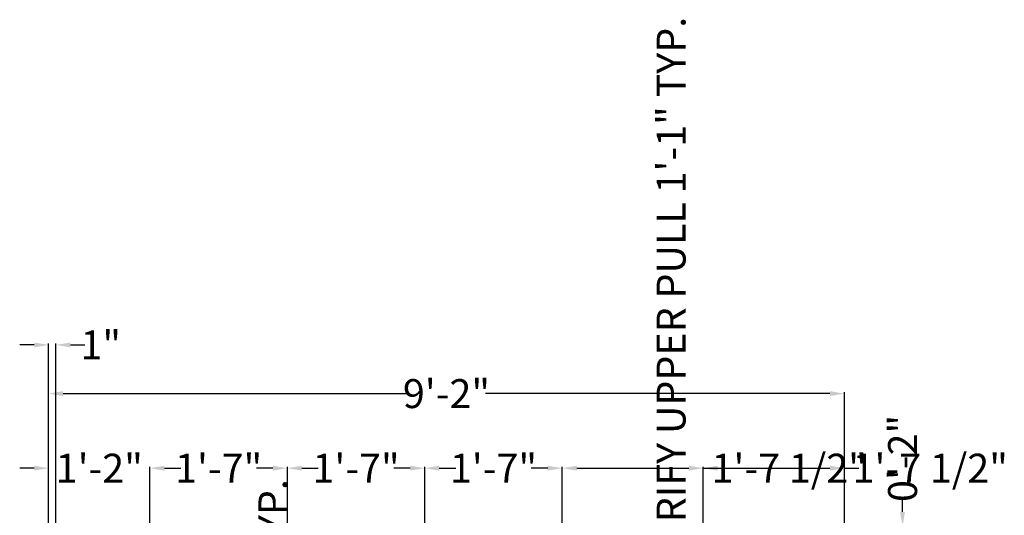
# Model space of a CAD drawing. Units: inches. Extents: x 13 to 156, y 156 to 357.
# Tile 3 of 3: x 20 to 156, y 289 to 357. Entities that reach past the tile are written whole.
import ezdxf

# ---------------------------------------------------------------- set-up
doc = ezdxf.new("R2010")
doc.units = ezdxf.units.IN
doc.header["$MEASUREMENT"] = 0
doc.layers.add('A-ANNO-DIMS', color=2, linetype='Continuous', lineweight=18)
doc.styles.get("Standard").update_dxf_attribs({"font": 'arial.ttf'})
doc.dimstyles.get("Standard").update_dxf_attribs({"dimtxt": 4, "dimasz": 2, "dimexe": 0.18, "dimexo": 0.0625, "dimgap": 0.09, "dimtad": 0, "dimdec": 0, "dimzin": 0, "dimdsep": 46, "dimlunit": 4, "dimtxsty": 'Standard', "dimcen": 0.09, "dimadec": 0, "dimazin": 0, "dimtfac": 1, "dimtdec": 0, "dimtofl": 0, "dimtmove": 0, "dimatfit": 3, "dimfxl": 1, "dimtolj": 1, "dimtzin": 0, "dimarcsym": 0})

# ---------------------------------------------------------------- blocks, each defined once
blk = doc.blocks.new('*D1')
at = {"layer": 'A-ANNO-DIMS', "color": 0, "lineweight": -2, "transparency": 16777216}
for p, q in [((23.63, 285.13), (23.63, 305.65)), ((25.63, 305.47), (73.22, 305.47)), ((131.63, 305.47), (84.03, 305.47)), ((133.63, 285.13), (133.63, 305.65))]:
    blk.add_line(p, q, dxfattribs=at)
at = {"layer": 'A-ANNO-DIMS', "color": 0, "transparency": 16777216}
for points in [[(25.63, 305.81), (25.63, 305.14), (23.63, 305.47)], [(131.63, 305.81), (131.63, 305.14), (133.63, 305.47)]]:
    blk.add_solid(points, dxfattribs=at)
at = {"layer": 'Defpoints', "color": 0, "transparency": 16777216}
for p in [(133.63, 305.47), (23.63, 285.07), (133.63, 285.07)]:
    blk.add_point(p, dxfattribs=at)
at = {"layer": 'A-ANNO-DIMS', "color": 0, "transparency": 16777216, "insert": (78.63, 305.47), "char_height": 4, "attachment_point": 5}
blk.add_mtext('\\A1;9\'-2"', dxfattribs=at)
blk = doc.blocks.new('*D2')
at = {"layer": 'A-ANNO-DIMS', "color": 0, "lineweight": -2, "transparency": 16777216}
for p, q in [((21.63, 312.2), (19.63, 312.2)), ((23.63, 285.13), (23.63, 312.38)), ((24.63, 285.13), (24.63, 312.38)), ((26.63, 312.2), (28.63, 312.2))]:
    blk.add_line(p, q, dxfattribs=at)
at = {"layer": 'A-ANNO-DIMS', "color": 0, "transparency": 16777216}
for points in [[(21.63, 312.54), (21.63, 311.87), (23.63, 312.2)], [(26.63, 312.54), (26.63, 311.87), (24.63, 312.2)]]:
    blk.add_solid(points, dxfattribs=at)
at = {"layer": 'Defpoints', "color": 0, "transparency": 16777216}
for p in [(24.63, 312.2), (23.63, 285.07), (24.63, 285.07)]:
    blk.add_point(p, dxfattribs=at)
at = {"layer": 'A-ANNO-DIMS', "color": 0, "transparency": 16777216, "insert": (30.83, 312.2), "char_height": 4, "attachment_point": 5}
blk.add_mtext('\\A1;1"', dxfattribs=at)
blk = doc.blocks.new('*D19')
at = {"layer": 'A-ANNO-DIMS', "color": 0, "lineweight": -2, "transparency": 16777216}
for p, q in [((109.68, 276.03), (109.68, 278.03)), ((111.56, 276.03), (109.5, 276.03)), ((109.68, 265.07), (109.68, 274.03)), ((111.56, 263.07), (109.5, 263.07))]:
    blk.add_line(p, q, dxfattribs=at)
at = {"layer": 'A-ANNO-DIMS', "color": 0, "transparency": 16777216}
for points in [[(109.35, 274.03), (110.01, 274.03), (109.68, 276.03)], [(109.35, 265.07), (110.01, 265.07), (109.68, 263.07)]]:
    blk.add_solid(points, dxfattribs=at)
at = {"layer": 'Defpoints', "color": 0, "transparency": 16777216}
for p in [(109.68, 276.03), (111.62, 276.03), (111.62, 263.07)]:
    blk.add_point(p, dxfattribs=at)
at = {"layer": 'A-ANNO-DIMS', "color": 0, "transparency": 16777216, "insert": (109.68, 319.45), "char_height": 4, "attachment_point": 5, "rotation": 90}
blk.add_mtext('\\A1;VERIFY UPPER PULL 1\'-1" TYP.', dxfattribs=at)
blk = doc.blocks.new('*D21')
at = {"layer": 'A-ANNO-DIMS', "color": 0, "lineweight": -2, "transparency": 16777216}
for p, q in [((54.63, 231.33), (54.63, 233.33)), ((58.13, 231.33), (54.45, 231.33)), ((54.63, 209.57), (54.63, 229.33)), ((58.13, 207.57), (54.45, 207.57))]:
    blk.add_line(p, q, dxfattribs=at)
at = {"layer": 'A-ANNO-DIMS', "color": 0, "transparency": 16777216}
for points in [[(54.29, 229.33), (54.96, 229.33), (54.63, 231.33)], [(54.29, 209.57), (54.96, 209.57), (54.63, 207.57)]]:
    blk.add_solid(points, dxfattribs=at)
at = {"layer": 'Defpoints', "color": 0, "transparency": 16777216}
for p in [(54.63, 231.33), (58.19, 231.33), (58.19, 207.57)]:
    blk.add_point(p, dxfattribs=at)
at = {"layer": 'A-ANNO-DIMS', "color": 0, "transparency": 16777216, "insert": (54.63, 264.31), "char_height": 4, "attachment_point": 5, "rotation": 90}
blk.add_mtext('\\A1;LOWER PULL 2\'-0" TYP.', dxfattribs=at)
blk = doc.blocks.new('*D31')
at = {"layer": 'A-ANNO-DIMS', "color": 0, "lineweight": -2, "transparency": 16777216}
for p, q in [((21.63, 295.16), (19.63, 295.16)), ((23.63, 285.13), (23.63, 295.34)), ((37.63, 285.13), (37.63, 295.34)), ((39.63, 295.16), (41.63, 295.16))]:
    blk.add_line(p, q, dxfattribs=at)
at = {"layer": 'A-ANNO-DIMS', "color": 0, "transparency": 16777216}
for points in [[(21.63, 295.49), (21.63, 294.82), (23.63, 295.16)], [(39.63, 295.49), (39.63, 294.82), (37.63, 295.16)]]:
    blk.add_solid(points, dxfattribs=at)
at = {"layer": 'Defpoints', "color": 0, "transparency": 16777216}
for p in [(37.63, 295.16), (23.63, 285.07), (37.63, 285.07)]:
    blk.add_point(p, dxfattribs=at)
at = {"layer": 'A-ANNO-DIMS', "color": 0, "transparency": 16777216, "insert": (30.63, 295.16), "char_height": 4, "attachment_point": 5}
blk.add_mtext('\\A1;1\'-2"', dxfattribs=at)
blk = doc.blocks.new('*D32')
at = {"layer": 'A-ANNO-DIMS', "color": 0, "lineweight": -2, "transparency": 16777216}
for p, q in [((37.63, 285.13), (37.63, 295.34)), ((39.63, 295.16), (41.91, 295.16)), ((54.63, 295.16), (52.35, 295.16)), ((56.63, 285.13), (56.63, 295.34))]:
    blk.add_line(p, q, dxfattribs=at)
at = {"layer": 'A-ANNO-DIMS', "color": 0, "transparency": 16777216}
for points in [[(39.63, 295.49), (39.63, 294.82), (37.63, 295.16)], [(54.63, 295.49), (54.63, 294.82), (56.63, 295.16)]]:
    blk.add_solid(points, dxfattribs=at)
at = {"layer": 'Defpoints', "color": 0, "transparency": 16777216}
for p in [(56.63, 295.16), (37.63, 285.07), (56.63, 285.07)]:
    blk.add_point(p, dxfattribs=at)
at = {"layer": 'A-ANNO-DIMS', "color": 0, "transparency": 16777216, "insert": (47.13, 295.16), "char_height": 4, "attachment_point": 5}
blk.add_mtext('\\A1;1\'-7"', dxfattribs=at)
blk = doc.blocks.new('*D33')
at = {"layer": 'A-ANNO-DIMS', "color": 0, "lineweight": -2, "transparency": 16777216}
for p, q in [((56.63, 285.13), (56.63, 295.34)), ((58.63, 295.16), (60.91, 295.16)), ((73.63, 295.16), (71.35, 295.16)), ((75.63, 285.13), (75.63, 295.34))]:
    blk.add_line(p, q, dxfattribs=at)
at = {"layer": 'A-ANNO-DIMS', "color": 0, "transparency": 16777216}
for points in [[(58.63, 295.49), (58.63, 294.82), (56.63, 295.16)], [(73.63, 295.49), (73.63, 294.82), (75.63, 295.16)]]:
    blk.add_solid(points, dxfattribs=at)
at = {"layer": 'Defpoints', "color": 0, "transparency": 16777216}
for p in [(75.63, 295.16), (56.63, 285.07), (75.63, 285.07)]:
    blk.add_point(p, dxfattribs=at)
at = {"layer": 'A-ANNO-DIMS', "color": 0, "transparency": 16777216, "insert": (66.13, 295.16), "char_height": 4, "attachment_point": 5}
blk.add_mtext('\\A1;1\'-7"', dxfattribs=at)
blk = doc.blocks.new('*D34')
at = {"layer": 'A-ANNO-DIMS', "color": 0, "lineweight": -2, "transparency": 16777216}
for p, q in [((75.63, 285.13), (75.63, 295.34)), ((77.63, 295.16), (79.91, 295.16)), ((92.63, 295.16), (90.35, 295.16)), ((94.63, 285.13), (94.63, 295.34))]:
    blk.add_line(p, q, dxfattribs=at)
at = {"layer": 'A-ANNO-DIMS', "color": 0, "transparency": 16777216}
for points in [[(77.63, 295.49), (77.63, 294.82), (75.63, 295.16)], [(92.63, 295.49), (92.63, 294.82), (94.63, 295.16)]]:
    blk.add_solid(points, dxfattribs=at)
at = {"layer": 'Defpoints', "color": 0, "transparency": 16777216}
for p in [(94.63, 295.16), (75.63, 285.07), (94.63, 285.07)]:
    blk.add_point(p, dxfattribs=at)
at = {"layer": 'A-ANNO-DIMS', "color": 0, "transparency": 16777216, "insert": (85.13, 295.16), "char_height": 4, "attachment_point": 5}
blk.add_mtext('\\A1;1\'-7"', dxfattribs=at)
blk = doc.blocks.new('*D35')
at = {"layer": 'A-ANNO-DIMS', "color": 0, "lineweight": -2, "transparency": 16777216}
for p, q in [((94.63, 285.13), (94.63, 295.34)), ((96.63, 295.16), (112.13, 295.16)), ((114.13, 285.13), (114.13, 295.34)), ((114.13, 295.16), (116.13, 295.16))]:
    blk.add_line(p, q, dxfattribs=at)
at = {"layer": 'A-ANNO-DIMS', "color": 0, "transparency": 16777216}
for points in [[(96.63, 295.49), (96.63, 294.82), (94.63, 295.16)], [(112.13, 295.49), (112.13, 294.82), (114.13, 295.16)]]:
    blk.add_solid(points, dxfattribs=at)
at = {"layer": 'Defpoints', "color": 0, "transparency": 16777216}
for p in [(114.13, 295.16), (94.63, 285.07), (114.13, 285.07)]:
    blk.add_point(p, dxfattribs=at)
at = {"layer": 'A-ANNO-DIMS', "color": 0, "transparency": 16777216, "insert": (126.01, 295.16), "char_height": 4, "attachment_point": 5}
blk.add_mtext('\\A1;1\'-7 1/2"', dxfattribs=at)
blk = doc.blocks.new('*D36')
at = {"layer": 'A-ANNO-DIMS', "color": 0, "lineweight": -2, "transparency": 16777216}
for p, q in [((114.13, 285.13), (114.13, 295.34)), ((116.13, 295.16), (131.63, 295.16)), ((133.63, 285.13), (133.63, 295.34)), ((133.63, 295.16), (135.63, 295.16))]:
    blk.add_line(p, q, dxfattribs=at)
at = {"layer": 'A-ANNO-DIMS', "color": 0, "transparency": 16777216}
for points in [[(116.13, 295.49), (116.13, 294.82), (114.13, 295.16)], [(131.63, 295.49), (131.63, 294.82), (133.63, 295.16)]]:
    blk.add_solid(points, dxfattribs=at)
at = {"layer": 'Defpoints', "color": 0, "transparency": 16777216}
for p in [(133.63, 295.16), (114.13, 285.07), (133.63, 285.07)]:
    blk.add_point(p, dxfattribs=at)
at = {"layer": 'A-ANNO-DIMS', "color": 0, "transparency": 16777216, "insert": (145.51, 295.16), "char_height": 4, "attachment_point": 5}
blk.add_mtext('\\A1;1\'-7 1/2"', dxfattribs=at)
blk = doc.blocks.new('*D37')
at = {"layer": 'A-ANNO-DIMS', "color": 0, "lineweight": -2, "transparency": 16777216}
for p, q in [((141.68, 289.11), (141.68, 291.11)), ((133.69, 287.11), (141.86, 287.11)), ((133.69, 285.07), (141.86, 285.07)), ((141.68, 283.07), (141.68, 281.07))]:
    blk.add_line(p, q, dxfattribs=at)
at = {"layer": 'A-ANNO-DIMS', "color": 0, "transparency": 16777216}
for points in [[(141.34, 289.11), (142.01, 289.11), (141.68, 287.11)], [(141.34, 283.07), (142.01, 283.07), (141.68, 285.07)]]:
    blk.add_solid(points, dxfattribs=at)
at = {"layer": 'Defpoints', "color": 0, "transparency": 16777216}
for p in [(133.63, 287.11), (141.68, 287.11), (133.63, 285.07)]:
    blk.add_point(p, dxfattribs=at)
at = {"layer": 'A-ANNO-DIMS', "color": 0, "transparency": 16777216, "insert": (141.68, 296.51), "char_height": 4, "attachment_point": 5, "rotation": 90}
blk.add_mtext('\\A1;0\'-2"', dxfattribs=at)

msp = doc.modelspace()

# ---------------------------------------------------------------- dimensions: what is measured, and where the dimension line sits
at = {"layer": 'A-ANNO-DIMS'}
for base, p1, p2, text, picture, middle in [((109.68, 276.03), (111.62, 263.07), (111.62, 276.03), 'VERIFY UPPER PULL <> TYP.', '*D19', (109.68, 319.45)), ((54.63, 231.33), (58.19, 207.57), (58.19, 231.33), 'LOWER PULL <> TYP.', '*D21', (54.63, 264.31))]:
    dim = msp.add_linear_dim(base=base, p1=p1, p2=p2, angle=90, text=text, dimstyle='Standard', override={"dimdec": 1, "dimlfac": 1, "dimrnd": 0, "dimzin": 1, "dimdsep": 46, "dimlunit": 4, "dimfrac": 2}, dxfattribs=at)
    dim.commit()
    dim.dimension.update_dxf_attribs({"geometry": picture, "text_midpoint": middle})
for base, p1, p2, override, picture, middle in [((24.63, 312.2), (23.63, 285.07), (24.63, 285.07), {"dimclrd": 0, "dimclre": 0, "dimclrt": 0}, '*D2', (30.83, 312.2)), ((133.63, 305.47), (23.63, 285.07), (133.63, 285.07), {"dimclrd": 0, "dimclre": 0, "dimclrt": 0}, '*D1', (78.63, 305.47)), ((114.13, 295.16), (94.63, 285.07), (114.13, 285.07), {"dimdec": 1, "dimlfac": 1, "dimrnd": 0, "dimzin": 1, "dimdsep": 46, "dimlunit": 4, "dimfrac": 2}, '*D35', (126.01, 295.16)), ((133.63, 295.16), (114.13, 285.07), (133.63, 285.07), {"dimdec": 1, "dimlfac": 1, "dimrnd": 0, "dimzin": 1, "dimdsep": 46, "dimlunit": 4, "dimfrac": 2}, '*D36', (145.51, 295.16)), ((37.63, 295.16), (23.63, 285.07), (37.63, 285.07), {"dimdec": 1, "dimlfac": 1, "dimrnd": 0, "dimzin": 1, "dimdsep": 46, "dimlunit": 4, "dimfrac": 2}, '*D31', (30.63, 295.16)), ((56.63, 295.16), (37.63, 285.07), (56.63, 285.07), {"dimdec": 1, "dimlfac": 1, "dimrnd": 0, "dimzin": 1, "dimdsep": 46, "dimlunit": 4, "dimfrac": 2}, '*D32', (47.13, 295.16)), ((75.63, 295.16), (56.63, 285.07), (75.63, 285.07), {"dimdec": 1, "dimlfac": 1, "dimrnd": 0, "dimzin": 1, "dimdsep": 46, "dimlunit": 4, "dimfrac": 2}, '*D33', (66.13, 295.16)), ((94.63, 295.16), (75.63, 285.07), (94.63, 285.07), {"dimdec": 1, "dimlfac": 1, "dimrnd": 0, "dimzin": 1, "dimdsep": 46, "dimlunit": 4, "dimfrac": 2}, '*D34', (85.13, 295.16))]:
    dim = msp.add_linear_dim(base=base, p1=p1, p2=p2, dimstyle='Standard', override=override, dxfattribs=at)
    dim.commit()
    dim.dimension.update_dxf_attribs({"geometry": picture, "text_midpoint": middle})
dim = msp.add_linear_dim(base=(141.68, 287.11), p1=(133.63, 285.07), p2=(133.63, 287.11), angle=90, dimstyle='Standard', override={"dimdec": 1, "dimlfac": 1, "dimrnd": 0, "dimzin": 1, "dimdsep": 46, "dimlunit": 4, "dimfrac": 2}, dxfattribs=at)
dim.commit()
dim.dimension.update_dxf_attribs({"geometry": '*D37', "text_midpoint": (141.68, 296.51)})

doc.saveas('drawing.dxf')
